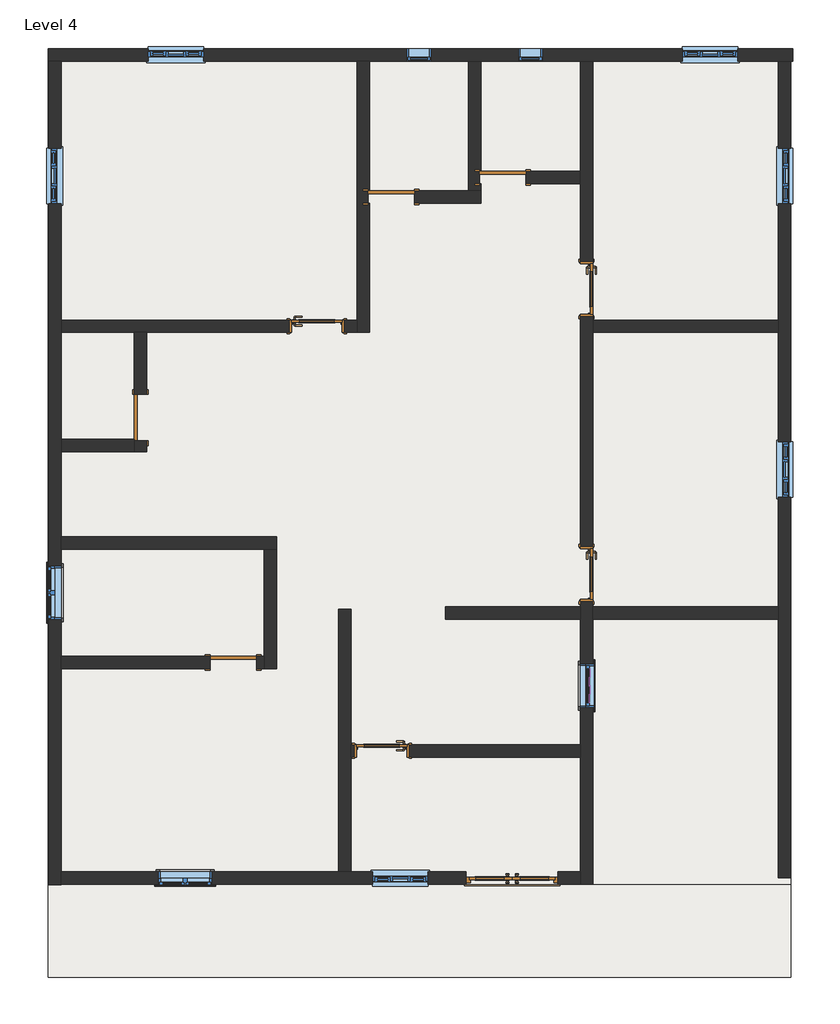
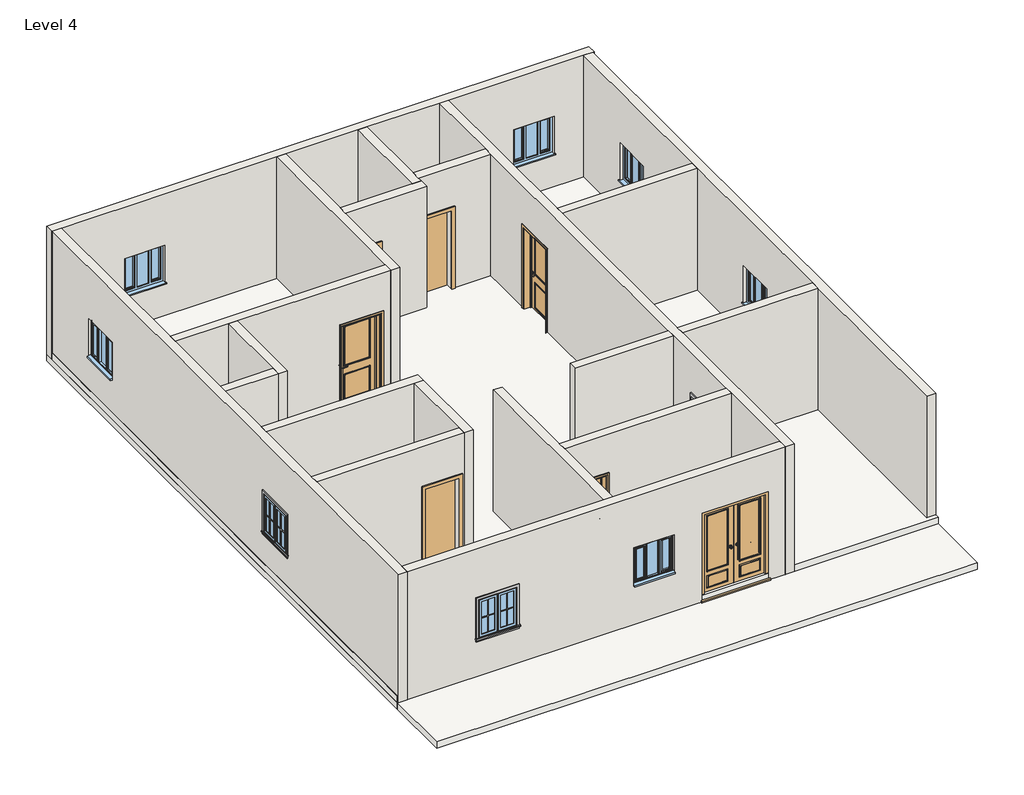
# One storey, incomplete: 19 walls, 12 proxies, 11 windows, 9 doors, 2 slabs, 1 roof.
"""IFC4 building model written with IfcOpenShell, lengths in millimetres."""

from ifc_helpers import new_model, si_unit, frame, origin, place, context, project, spatial, polyline, outline, extrude, faceted_brep, transform, mapped, element, save
from components import muntin_pattern_2x2_muntin_pattern_2x2_b3fe6957, muntin_pattern_2x2_muntin_pattern_2x2_3e0ecaf2, muntin_pattern_2x2_muntin_pattern_2x2_5f474966, trim_window_exterior_flat_with_sill_41619996, trim_window_exterior_flat_with_sill_68241f6a, trim_window_interior_flat_picture_frame_51c85655, trim_window_interior_flat_picture_frame_d3d93820, doors_extdbl_w_glazing_bars_2_1510x2110mm_e5cd3545, doors_extdbl_w_glazing_bars_2_1510x2110mm_b3535315, doors_intsgl_w_transome_910x2110mm_1071bad6, doors_intsgl_w_transome_910x2110mm_0d7ac49b, door_fadea3f2, door_53b1b562, window_085f26e1, window_c29befe5, window_4d695ea9, windows_tpl_plain_910x910mm_84e79c20

model = new_model("IFC4")

# Units and contexts
model_context = context("Model", 3, world=origin())
ifc_project = project(units=[si_unit("LENGTHUNIT", "METRE", prefix="MILLI")], contexts=[model_context])

# Site, building, storey
site = spatial("IfcSite", under=ifc_project)
building = spatial("IfcBuilding", under=site)
storey = spatial("IfcBuildingStorey", under=building, Name="Level 4", Elevation=9144.0)

# Proxies
placement = place(None, origin())
muntin_pattern_2x2_muntin_pattern_2x2_shape = muntin_pattern_2x2_muntin_pattern_2x2_b3fe6957(model_context)
element("IfcBuildingElementProxy", 1, Name="Muntin Pattern_2x2 : Muntin Pattern_2x2", ObjectType="Muntin Pattern_2x2 : Muntin Pattern_2x2", at=placement, inside=storey, context=model_context, shape_type="MappedRepresentation", body=[
    mapped(muntin_pattern_2x2_muntin_pattern_2x2_shape, transform((-4444.3565281, -6259.9254533, 10128.25), x_axis=(-1.0, 0.0, 0.0), y_axis=(0.0, -1.0, 0.0), z_axis=(0.0, 0.0, 1.0))),
])
element("IfcBuildingElementProxy", 2, Name="Muntin Pattern_2x2 : Muntin Pattern_2x2", ObjectType="Muntin Pattern_2x2 : Muntin Pattern_2x2", at=placement, inside=storey, context=model_context, shape_type="MappedRepresentation", body=[
    mapped(muntin_pattern_2x2_muntin_pattern_2x2_shape, transform((-6884.3440281, -1708.5629533, 10128.25), x_axis=(0.0, 1.0, 0.0), y_axis=(-1.0, 0.0, 0.0), z_axis=(0.0, 0.0, 1.0))),
])
muntin_pattern_2x2_muntin_pattern_2x2_2_shape = muntin_pattern_2x2_muntin_pattern_2x2_3e0ecaf2(model_context)
element("IfcBuildingElementProxy", 3, Name="Muntin Pattern_2x2 : Muntin Pattern_2x2", ObjectType="Muntin Pattern_2x2 : Muntin Pattern_2x2", at=placement, inside=storey, context=model_context, shape_type="MappedRepresentation", body=[
    mapped(muntin_pattern_2x2_muntin_pattern_2x2_2_shape, transform((-4872.9815281, -6259.9254533, 10128.25), x_axis=(1.0, 0.0, 0.0), y_axis=(0.0, 1.0, 0.0), z_axis=(0.0, 0.0, 1.0))),
])
element("IfcBuildingElementProxy", 4, Name="Muntin Pattern_2x2 : Muntin Pattern_2x2", ObjectType="Muntin Pattern_2x2 : Muntin Pattern_2x2", at=placement, inside=storey, context=model_context, shape_type="MappedRepresentation", body=[
    mapped(muntin_pattern_2x2_muntin_pattern_2x2_2_shape, transform((-6884.3440281, -1279.9379533, 10128.25), x_axis=(0.0, -1.0, 0.0), y_axis=(1.0, 0.0, 0.0), z_axis=(0.0, 0.0, 1.0))),
])
muntin_pattern_2x2_muntin_pattern_2x2_3_shape = muntin_pattern_2x2_muntin_pattern_2x2_5f474966(model_context)
element("IfcBuildingElementProxy", 5, Name="Muntin Pattern_2x2 : Muntin Pattern_2x2", ObjectType="Muntin Pattern_2x2 : Muntin Pattern_2x2", at=placement, inside=storey, context=model_context, shape_type="MappedRepresentation", body=[
    mapped(muntin_pattern_2x2_muntin_pattern_2x2_3_shape, transform((1989.809459, -3018.2504533, 10664.825), x_axis=(0.0, -1.0, 0.0), y_axis=(1.0, 0.0, 0.0), z_axis=(0.0, 0.0, 1.0))),
])
element("IfcBuildingElementProxy", 6, Name="Muntin Pattern_2x2 : Muntin Pattern_2x2", ObjectType="Muntin Pattern_2x2 : Muntin Pattern_2x2", at=placement, inside=storey, context=model_context, shape_type="MappedRepresentation", body=[
    mapped(muntin_pattern_2x2_muntin_pattern_2x2_3_shape, transform((1945.359459, -3018.2504533, 10134.6), x_axis=(0.0, -1.0, 0.0), y_axis=(1.0, 0.0, 0.0), z_axis=(0.0, 0.0, 1.0))),
])
trim_window_exterior_flat_with_sill_shape = trim_window_exterior_flat_with_sill_41619996(model_context)
element("IfcBuildingElementProxy", 7, Name="Trim-Window-Exterior-Flat : with Sill", ObjectType="Trim-Window-Exterior-Flat : with Sill", at=placement, inside=storey, context=model_context, shape_type="MappedRepresentation", body=[
    mapped(trim_window_exterior_flat_with_sill_shape, transform((-4658.6690281, -6269.4504533, 10972.8), x_axis=(1.0, 0.0, 0.0), y_axis=(0.0, 0.0, 1.0), z_axis=(0.0, -1.0, 0.0))),
])
element("IfcBuildingElementProxy", 8, Name="Trim-Window-Exterior-Flat : with Sill", ObjectType="Trim-Window-Exterior-Flat : with Sill", at=placement, inside=storey, context=model_context, shape_type="MappedRepresentation", body=[
    mapped(trim_window_exterior_flat_with_sill_shape, transform((-6893.8690281, -1494.2504533, 10972.8), x_axis=(0.0, -1.0, 0.0), y_axis=(0.0, 0.0, 1.0), z_axis=(-1.0, 0.0, 0.0))),
])
trim_window_exterior_flat_with_sill_2_shape = trim_window_exterior_flat_with_sill_68241f6a(model_context)
element("IfcBuildingElementProxy", 9, Name="Trim-Window-Exterior-Flat : with Sill", ObjectType="Trim-Window-Exterior-Flat : with Sill", at=placement, inside=storey, context=model_context, shape_type="MappedRepresentation", body=[
    mapped(trim_window_exterior_flat_with_sill_2_shape, transform((2024.734459, -3018.2504533, 11226.8), x_axis=(0.0, 1.0, 0.0), y_axis=(0.0, 0.0, 1.0), z_axis=(1.0, 0.0, 0.0))),
])
trim_window_interior_flat_picture_frame_shape = trim_window_interior_flat_picture_frame_51c85655(model_context)
element("IfcBuildingElementProxy", 10, Name="Trim-Window-Interior-Flat : Picture Frame", ObjectType="Trim-Window-Interior-Flat : Picture Frame", at=placement, inside=storey, context=model_context, shape_type="MappedRepresentation", body=[
    mapped(trim_window_interior_flat_picture_frame_shape, transform((-4658.6690281, -6066.2504533, 10972.8), x_axis=(-1.0, 0.0, 0.0), y_axis=(0.0, 0.0, 1.0), z_axis=(0.0, 1.0, 0.0))),
])
element("IfcBuildingElementProxy", 11, Name="Trim-Window-Interior-Flat : Picture Frame", ObjectType="Trim-Window-Interior-Flat : Picture Frame", at=placement, inside=storey, context=model_context, shape_type="MappedRepresentation", body=[
    mapped(trim_window_interior_flat_picture_frame_shape, transform((-6690.6690281, -1494.2504533, 10972.8), x_axis=(0.0, 1.0, 0.0), y_axis=(0.0, 0.0, 1.0), z_axis=(1.0, 0.0, 0.0))),
])
trim_window_interior_flat_picture_frame_2_shape = trim_window_interior_flat_picture_frame_d3d93820(model_context)
element("IfcBuildingElementProxy", 12, Name="Trim-Window-Interior-Flat : Picture Frame", ObjectType="Trim-Window-Interior-Flat : Picture Frame", at=placement, inside=storey, context=model_context, shape_type="MappedRepresentation", body=[
    mapped(trim_window_interior_flat_picture_frame_2_shape, transform((1821.534459, -3018.2504533, 11226.8), x_axis=(0.0, -1.0, 0.0), y_axis=(0.0, 0.0, 1.0), z_axis=(-1.0, 0.0, 0.0))),
])

# Doors
doors_extdbl_w_glazing_bars_2_1510x2110mm_shape = doors_extdbl_w_glazing_bars_2_1510x2110mm_e5cd3545(model_context)
doors_extdbl_w_glazing_bars_2_1510x2110mm_2_shape = doors_extdbl_w_glazing_bars_2_1510x2110mm_b3535315(model_context)
element("IfcDoor", 13, ObjectType="Doors_ExtDbl_w-Glazing_Bars_2 : 1510x2110mm", at=placement, inside=storey, context=model_context, shape_type="MappedRepresentation", body=[
    mapped(doors_extdbl_w_glazing_bars_2_1510x2110mm_shape, transform((703.934459, -6167.8504533, 9144.0), x_axis=(-1.0, 0.0, 0.0), y_axis=(0.0, -1.0, 0.0), z_axis=(0.0, 0.0, 1.0))),
    mapped(doors_extdbl_w_glazing_bars_2_1510x2110mm_2_shape, transform((703.934459, -6167.8504533, 9144.0), x_axis=(-1.0, 0.0, 0.0), y_axis=(0.0, -1.0, 0.0), z_axis=(0.0, 0.0, 1.0))),
])
doors_intsgl_w_transome_910x2110mm_shape = doors_intsgl_w_transome_910x2110mm_1071bad6(model_context)
element("IfcDoor", 14, ObjectType="Doors_IntSgl_w-Transome : 910x2110mm", at=placement, inside=storey, context=model_context, shape_type="MappedRepresentation", body=[
    mapped(doors_intsgl_w_transome_910x2110mm_shape, transform((-1432.8690281, -4085.0504533, 9144.0), x_axis=(-1.0, 0.0, 0.0), y_axis=(0.0, -1.0, 0.0), z_axis=(0.0, 0.0, 1.0))),
])
doors_intsgl_w_transome_910x2110mm_2_shape = doors_intsgl_w_transome_910x2110mm_0d7ac49b(model_context)
element("IfcDoor", 15, ObjectType="Doors_IntSgl_w-Transome : 910x2110mm", at=placement, inside=storey, context=model_context, shape_type="MappedRepresentation", body=[
    mapped(doors_intsgl_w_transome_910x2110mm_2_shape, transform((-2499.6690281, 2874.5495467, 9144.0), x_axis=(1.0, 0.0, 0.0), y_axis=(0.0, 1.0, 0.0), z_axis=(0.0, 0.0, 1.0))),
])
element("IfcDoor", 16, ObjectType="Doors_IntSgl_w-Transome : 910x2110mm", at=placement, inside=storey, context=model_context, shape_type="MappedRepresentation", body=[
    mapped(doors_intsgl_w_transome_910x2110mm_2_shape, transform((1923.134459, 3484.1495467, 9144.0), x_axis=(0.0, -1.0, 0.0), y_axis=(1.0, 0.0, 0.0), z_axis=(0.0, 0.0, 1.0))),
])
element("IfcDoor", 17, ObjectType="Doors_IntSgl_w-Transome : 910x2110mm", at=placement, inside=storey, context=model_context, shape_type="MappedRepresentation", body=[
    mapped(doors_intsgl_w_transome_910x2110mm_2_shape, transform((1923.134459, -1189.4504533, 9144.0), x_axis=(0.0, -1.0, 0.0), y_axis=(1.0, 0.0, 0.0), z_axis=(0.0, 0.0, 1.0))),
])
door_shape = door_fadea3f2(model_context)
element("IfcDoor", 18, ObjectType="Single-Flush : 30\" x 80\"", at=placement, inside=storey, context=model_context, shape_type="MappedRepresentation", body=[
    mapped(door_shape, transform((-3871.2690281, -2637.2504533, 9144.0), x_axis=(1.0, 0.0, 0.0), y_axis=(0.0, 1.0, 0.0), z_axis=(0.0, 0.0, 1.0))),
])
door_2_shape = door_53b1b562(model_context)
element("IfcDoor", 19, ObjectType="Single-Flush : 30\" x 80\"", at=placement, inside=storey, context=model_context, shape_type="MappedRepresentation", body=[
    mapped(door_2_shape, transform((-5395.2690281, 1375.9495467, 9144.0), x_axis=(0.0, -1.0, 0.0), y_axis=(1.0, 0.0, 0.0), z_axis=(0.0, 0.0, 1.0))),
])
element("IfcDoor", 20, ObjectType="Single-Flush : 30\" x 80\"", at=placement, inside=storey, context=model_context, shape_type="MappedRepresentation", body=[
    mapped(door_2_shape, transform((-1280.4690281, 4995.4495467, 9144.0), x_axis=(-1.0, 0.0, 0.0), y_axis=(0.0, -1.0, 0.0), z_axis=(0.0, 0.0, 1.0))),
])
element("IfcDoor", 21, ObjectType="Single-Flush : 30\" x 80\"", at=placement, inside=storey, context=model_context, shape_type="MappedRepresentation", body=[
    mapped(door_2_shape, transform((548.3309719, 5312.9495467, 9144.0), x_axis=(-1.0, 0.0, 0.0), y_axis=(0.0, -1.0, 0.0), z_axis=(0.0, 0.0, 1.0))),
])

# Roof
element("IfcRoof", 22, ObjectType="Generic - 12\"", at=placement, inside=storey, context=model_context, shape_type="SweptSolid", body=[
    extrude(outline(polyline([(-6906.5690281, 7421.1495467), (5272.7309719, 7421.1495467), (5272.7309719, -6269.4504533), (-6906.5690281, -6269.4504533), (-6906.5690281, 7421.1495467)])), frame((0.0, 0.0, 9144.0), z_axis=(0.0, 0.0, 1.0), x_axis=(1.0, 0.0, 0.0)), (0.0, 0.0, 1.0), 152.4),
])

# Slabs
element("IfcSlab", 23, ObjectType="Generic - 12\"", at=placement, inside=storey, context=model_context, shape_type="SweptSolid", body=[
    extrude(outline(polyline([(5272.7309719, 7421.1495467), (5272.7309719, -6269.4504533), (-6906.5690281, -6269.4504533), (-6906.5690281, 7421.1495467), (5272.7309719, 7421.1495467)])), frame((0.0, 0.0, 8991.6), z_axis=(0.0, 0.0, 1.0), x_axis=(1.0, 0.0, 0.0)), (0.0, 0.0, 1.0), 152.4),
])
element("IfcSlab", 24, ObjectType="Generic - 12\"", at=placement, inside=storey, context=model_context, shape_type="SweptSolid", body=[
    extrude(outline(polyline([(5272.7309719, -6269.4504533), (5272.7309719, -7799.0240652), (-6906.5690281, -7799.0240652), (-6906.5690281, -6269.4504533), (5272.7309719, -6269.4504533)])), frame((0.0, 0.0, 8991.6), z_axis=(0.0, 0.0, 1.0), x_axis=(1.0, 0.0, 0.0)), (0.0, 0.0, 1.0), 152.4),
])

# Walls
element("IfcWall", 25, ObjectType="4.5\" p", at=placement, inside=storey, context=model_context, shape_type="Brep", body=[
    faceted_brep([(-1839.2690281, 7217.9495467, 9144.0), (-1839.2690281, 2976.1495467, 9144.0), (-1839.2690281, 2772.9495467, 9144.0), (-1839.2690281, 2772.9495467, 12192.0), (-1839.2690281, 2976.1495467, 12192.0), (-1839.2690281, 7217.9495467, 12192.0), (-1636.0690281, 7217.9495467, 12192.0), (-1636.0690281, 5097.0495467, 12192.0), (-1636.0690281, 4893.8495467, 12192.0), (-1636.0690281, 2772.9495467, 12192.0), (-1636.0690281, 2772.9495467, 9144.0), (-1636.0690281, 4893.8495467, 9144.0), (-1636.0690281, 4893.8495467, 11176.0), (-1636.0690281, 5097.0495467, 11176.0), (-1636.0690281, 5097.0495467, 9144.0), (-1636.0690281, 7217.9495467, 9144.0), (-1661.4690281, 5097.0495467, 9144.0), (-1661.4690281, 4893.8495467, 9144.0), (-1661.4690281, 5097.0495467, 11176.0), (-1661.4690281, 4893.8495467, 11176.0)], [[[0, 1, 2, 3, 4, 5]], [[6, 7, 8, 9, 10, 11, 12, 13, 14, 15]], [[2, 1, 0, 15, 14, 16, 17, 11, 10]], [[5, 4, 3, 9, 8, 7, 6]], [[0, 5, 6, 15]], [[3, 2, 10, 9]], [[18, 16, 14, 13]], [[17, 19, 12, 11]], [[19, 18, 13, 12]], [[16, 18, 19, 17]]]),
])
element("IfcWall", 26, ObjectType="4.5\" p", at=placement, inside=storey, context=model_context, shape_type="Brep", body=[
    faceted_brep([(-1839.2690281, 2772.9495467, 12192.0), (-5293.6690281, 2772.9495467, 12192.0), (-5496.8690281, 2772.9495467, 12192.0), (-6690.6690281, 2772.9495467, 12192.0), (-6690.6690281, 2772.9495467, 9144.0), (-5496.8690281, 2772.9495467, 9144.0), (-5293.6690281, 2772.9495467, 9144.0), (-2954.6690281, 2772.9495467, 9144.0), (-2954.6690281, 2772.9495467, 11254.0), (-2044.6690281, 2772.9495467, 11254.0), (-2044.6690281, 2772.9495467, 9144.0), (-1839.2690281, 2772.9495467, 9144.0), (-6690.6690281, 2976.1495467, 12192.0), (-1839.2690281, 2976.1495467, 12192.0), (-1839.2690281, 2976.1495467, 9144.0), (-2044.6690281, 2976.1495467, 9144.0), (-2044.6690281, 2976.1495467, 11254.0), (-2954.6690281, 2976.1495467, 11254.0), (-2954.6690281, 2976.1495467, 9144.0), (-6690.6690281, 2976.1495467, 9144.0)], [[[0, 1, 2, 3, 4, 5, 6, 7, 8, 9, 10, 11]], [[12, 13, 14, 15, 16, 17, 18, 19]], [[4, 19, 18, 7, 6, 5]], [[14, 11, 10, 15]], [[3, 2, 1, 0, 13, 12]], [[0, 11, 14, 13]], [[4, 3, 12, 19]], [[9, 16, 15, 10]], [[16, 9, 8, 17]], [[17, 8, 7, 18]]]),
])
element("IfcWall", 27, ObjectType="4.5\" p", at=placement, inside=storey, context=model_context, shape_type="Brep", body=[
    faceted_brep([(-5496.8690281, 994.9495467, 11176.0), (-5496.8690281, 994.9495467, 9144.0), (-5496.8690281, 817.1495467, 9144.0), (-5496.8690281, 817.1495467, 12192.0), (-5496.8690281, 1020.3495467, 12192.0), (-5496.8690281, 2772.9495467, 12192.0), (-5496.8690281, 2772.9495467, 9144.0), (-5496.8690281, 1756.9495467, 9144.0), (-5496.8690281, 1756.9495467, 11176.0), (-5293.6690281, 817.1495467, 9144.0), (-5293.6690281, 994.9495467, 9144.0), (-5293.6690281, 994.9495467, 11176.0), (-5293.6690281, 1756.9495467, 11176.0), (-5293.6690281, 1756.9495467, 9144.0), (-5293.6690281, 2772.9495467, 9144.0), (-5293.6690281, 2772.9495467, 12192.0), (-5293.6690281, 817.1495467, 12192.0)], [[[0, 1, 2, 3, 4, 5, 6, 7, 8]], [[9, 10, 11, 12, 13, 14, 15, 16]], [[7, 6, 14, 13]], [[2, 1, 10, 9]], [[5, 4, 3, 16, 15]], [[6, 5, 15, 14]], [[3, 2, 9, 16]], [[11, 10, 1, 0]], [[12, 11, 0, 8]], [[13, 12, 8, 7]]]),
])
element("IfcWall", 28, ObjectType="4.5\" p", at=placement, inside=storey, context=model_context, shape_type="SweptSolid", body=[
    extrude(outline(polyline([(-5496.8690281, 817.1495467), (-6690.6690281, 817.1495467), (-6690.6690281, 1020.3495467), (-5496.8690281, 1020.3495467), (-5496.8690281, 817.1495467)])), frame((0.0, 0.0, 9144.0), z_axis=(0.0, 0.0, 1.0), x_axis=(1.0, 0.0, 0.0)), (0.0, 0.0, 1.0), 3048.0),
])
element("IfcWall", 29, ObjectType="4.5\" p", at=placement, inside=storey, context=model_context, shape_type="Brep", body=[
    faceted_brep([(-6690.6690281, -783.0504533, 9144.0), (-3363.2690281, -783.0504533, 9144.0), (-3160.0690281, -783.0504533, 9144.0), (-3160.0690281, -783.0504533, 12192.0), (-3363.2690281, -783.0504533, 12192.0), (-6690.6690281, -783.0504533, 12192.0), (-6690.6690281, -579.8504533, 9144.0), (-6690.6690281, -579.8504533, 12192.0), (-3160.0690281, -579.8504533, 12192.0), (-3160.0690281, -579.8504533, 9144.0)], [[[0, 1, 2, 3, 4, 5]], [[6, 7, 8, 9]], [[2, 1, 0, 6, 9]], [[5, 4, 3, 8, 7]], [[0, 5, 7, 6]], [[3, 2, 9, 8]]]),
])
element("IfcWall", 30, ObjectType="4.5\" p", at=placement, inside=storey, context=model_context, shape_type="Brep", body=[
    faceted_brep([(-3363.2690281, -783.0504533, 9144.0), (-3363.2690281, -2535.6504533, 9144.0), (-3363.2690281, -2738.8504533, 9144.0), (-3363.2690281, -2738.8504533, 12192.0), (-3363.2690281, -2535.6504533, 12192.0), (-3363.2690281, -783.0504533, 12192.0), (-3160.0690281, -783.0504533, 9144.0), (-3160.0690281, -783.0504533, 12192.0), (-3160.0690281, -2738.8504533, 12192.0), (-3160.0690281, -2738.8504533, 9144.0)], [[[0, 1, 2, 3, 4, 5]], [[6, 7, 8, 9]], [[2, 1, 0, 6, 9]], [[5, 4, 3, 8, 7]], [[0, 5, 7, 6]], [[3, 2, 9, 8]]]),
])
element("IfcWall", 31, ObjectType="4.5\" p", at=placement, inside=storey, context=model_context, shape_type="SweptSolid", body=[
    extrude(outline(polyline([(11176.0, -3490.2690281), (9144.0, -3490.2690281), (9144.0, -3363.2690281), (12192.0, -3363.2690281), (12192.0, -6690.6690281), (9144.0, -6690.6690281), (9144.0, -4252.2690281), (11176.0, -4252.2690281), (11176.0, -3490.2690281)])), frame((0.0, -2738.8504533, 0.0), z_axis=(0.0, 1.0, 0.0), x_axis=(0.0, 0.0, 1.0)), (0.0, 0.0, 1.0), 203.2),
])
element("IfcWall", 32, ObjectType="4.5\" p", at=placement, inside=storey, context=model_context, shape_type="Brep", body=[
    faceted_brep([(192.7309719, 4893.8495467, 12192.0), (-1636.0690281, 4893.8495467, 12192.0), (-1636.0690281, 4893.8495467, 11176.0), (-899.4690281, 4893.8495467, 11176.0), (-899.4690281, 4893.8495467, 9144.0), (192.7309719, 4893.8495467, 9144.0), (-1636.0690281, 5097.0495467, 12192.0), (-10.4690281, 5097.0495467, 12192.0), (192.7309719, 5097.0495467, 12192.0), (192.7309719, 5097.0495467, 9144.0), (-10.4690281, 5097.0495467, 9144.0), (-899.4690281, 5097.0495467, 9144.0), (-899.4690281, 5097.0495467, 11176.0), (-1636.0690281, 5097.0495467, 11176.0)], [[[0, 1, 2, 3, 4, 5]], [[6, 7, 8, 9, 10, 11, 12, 13]], [[9, 5, 4, 11, 10]], [[1, 0, 8, 7, 6]], [[1, 6, 13, 2]], [[0, 5, 9, 8]], [[12, 3, 2, 13]], [[3, 12, 11, 4]]]),
])
element("IfcWall", 33, ObjectType="4.5\" p", at=placement, inside=storey, context=model_context, shape_type="Brep", body=[
    faceted_brep([(-10.4690281, 7217.9495467, 9144.0), (-10.4690281, 5097.0495467, 9144.0), (-10.4690281, 5097.0495467, 12192.0), (-10.4690281, 7217.9495467, 12192.0), (192.7309719, 7217.9495467, 12192.0), (192.7309719, 5414.5495467, 12192.0), (192.7309719, 5211.3495467, 12192.0), (192.7309719, 5097.0495467, 12192.0), (192.7309719, 5097.0495467, 9144.0), (192.7309719, 5211.3495467, 9144.0), (192.7309719, 5211.3495467, 11176.0), (192.7309719, 5414.5495467, 11176.0), (192.7309719, 5414.5495467, 9144.0), (192.7309719, 7217.9495467, 9144.0), (167.3309719, 5414.5495467, 9144.0), (167.3309719, 5211.3495467, 9144.0), (167.3309719, 5414.5495467, 11176.0), (167.3309719, 5211.3495467, 11176.0)], [[[0, 1, 2, 3]], [[4, 5, 6, 7, 8, 9, 10, 11, 12, 13]], [[1, 0, 13, 12, 14, 15, 9, 8]], [[3, 2, 7, 6, 5, 4]], [[2, 1, 8, 7]], [[0, 3, 4, 13]], [[16, 14, 12, 11]], [[15, 17, 10, 9]], [[17, 16, 11, 10]], [[14, 16, 17, 15]]]),
])
element("IfcWall", 34, ObjectType="4.5\" p", at=placement, inside=storey, context=model_context, shape_type="Brep", body=[
    faceted_brep([(1821.534459, -6269.4504533, 12192.0), (1821.534459, -6066.2504533, 12192.0), (1821.534459, -4186.6504533, 12192.0), (1821.534459, -3983.4504533, 12192.0), (1821.534459, -1926.0504533, 12192.0), (1821.534459, -1722.8504533, 12192.0), (1821.534459, 5211.3495467, 12192.0), (1821.534459, 5414.5495467, 12192.0), (1821.534459, 7217.9495467, 12192.0), (1821.534459, 7217.9495467, 9144.0), (1821.534459, 5414.5495467, 9144.0), (1821.534459, 5211.3495467, 9144.0), (1821.534459, 3939.1495467, 9144.0), (1821.534459, 3939.1495467, 11254.0), (1821.534459, 3029.1495467, 11254.0), (1821.534459, 3029.1495467, 9144.0), (1821.534459, -734.4504533, 9144.0), (1821.534459, -734.4504533, 11254.0), (1821.534459, -1644.4504533, 11254.0), (1821.534459, -1644.4504533, 9144.0), (1821.534459, -1722.8504533, 9144.0), (1821.534459, -1926.0504533, 9144.0), (1821.534459, -3983.4504533, 9144.0), (1821.534459, -4186.6504533, 9144.0), (1821.534459, -6066.2504533, 9144.0), (1821.534459, -6269.4504533, 9144.0), (1821.534459, -2662.6504533, 11226.8), (1821.534459, -3373.8504533, 11226.8), (1821.534459, -3373.8504533, 10058.4), (1821.534459, -2662.6504533, 10058.4), (2024.734459, 7217.9495467, 12192.0), (2024.734459, 2976.1495467, 12192.0), (2024.734459, 2772.9495467, 12192.0), (2024.734459, -1722.8504533, 12192.0), (2024.734459, -1926.0504533, 12192.0), (2024.734459, -6269.4504533, 12192.0), (2024.734459, -6269.4504533, 9144.0), (2024.734459, -1926.0504533, 9144.0), (2024.734459, -1722.8504533, 9144.0), (2024.734459, -1644.4504533, 9144.0), (2024.734459, -1644.4504533, 11254.0), (2024.734459, -734.4504533, 11254.0), (2024.734459, -734.4504533, 9144.0), (2024.734459, 2772.9495467, 9144.0), (2024.734459, 2976.1495467, 9144.0), (2024.734459, 3029.1495467, 9144.0), (2024.734459, 3029.1495467, 11254.0), (2024.734459, 3939.1495467, 11254.0), (2024.734459, 3939.1495467, 9144.0), (2024.734459, 7217.9495467, 9144.0), (2024.734459, -2662.6504533, 11226.8), (2024.734459, -2662.6504533, 10058.4), (2024.734459, -3373.8504533, 10058.4), (2024.734459, -3373.8504533, 11226.8)], [[[0, 1, 2, 3, 4, 5, 6, 7, 8, 9, 10, 11, 12, 13, 14, 15, 16, 17, 18, 19, 20, 21, 22, 23, 24, 25], [26, 27, 28, 29]], [[30, 31, 32, 33, 34, 35, 36, 37, 38, 39, 40, 41, 42, 43, 44, 45, 46, 47, 48, 49], [50, 51, 52, 53]], [[9, 49, 48, 12, 11, 10]], [[15, 45, 44, 43, 42, 16]], [[36, 25, 24, 23, 22, 21, 20, 19, 39, 38, 37]], [[8, 7, 6, 5, 4, 3, 2, 1, 0, 35, 34, 33, 32, 31, 30]], [[9, 8, 30, 49]], [[14, 46, 45, 15]], [[46, 14, 13, 47]], [[47, 13, 12, 48]], [[18, 40, 39, 19]], [[40, 18, 17, 41]], [[41, 17, 16, 42]], [[0, 25, 36, 35]], [[51, 50, 26, 29]], [[52, 51, 29, 28]], [[53, 52, 28, 27]], [[50, 53, 27, 26]]]),
])
element("IfcWall", 35, ObjectType="4.5\" p", at=placement, inside=storey, context=model_context, shape_type="SweptSolid", body=[
    extrude(outline(polyline([(-391.4690281, -1926.0504533), (-391.4690281, -1722.8504533), (1821.534459, -1722.8504533), (1821.534459, -1926.0504533), (-391.4690281, -1926.0504533)])), frame((0.0, 0.0, 9144.0), z_axis=(0.0, 0.0, 1.0), x_axis=(1.0, 0.0, 0.0)), (0.0, 0.0, 1.0), 3048.0),
    extrude(outline(polyline([(5069.5309719, -1722.8504533), (5069.5309719, -1926.0504533), (2024.734459, -1926.0504533), (2024.734459, -1722.8504533), (5069.5309719, -1722.8504533)])), frame((0.0, 0.0, 9144.0), z_axis=(0.0, 0.0, 1.0), x_axis=(1.0, 0.0, 0.0)), (0.0, 0.0, 1.0), 3048.0),
])
element("IfcWall", 36, ObjectType="4.5\" p", at=placement, inside=storey, context=model_context, shape_type="SweptSolid", body=[
    extrude(outline(polyline([(5069.5309719, 2772.9495467), (2024.734459, 2772.9495467), (2024.734459, 2976.1495467), (5069.5309719, 2976.1495467), (5069.5309719, 2772.9495467)])), frame((0.0, 0.0, 9144.0), z_axis=(0.0, 0.0, 1.0), x_axis=(1.0, 0.0, 0.0)), (0.0, 0.0, 1.0), 3048.0),
])
element("IfcWall", 37, ObjectType="4.5\" p", at=placement, inside=storey, context=model_context, shape_type="SweptSolid", body=[
    extrude(outline(polyline([(12192.0, 1821.534459), (12192.0, 192.7309719), (11176.0, 192.7309719), (11176.0, 929.3309719), (9144.0, 929.3309719), (9144.0, 1821.534459), (12192.0, 1821.534459)])), frame((0.0, 5211.3495467, 0.0), z_axis=(0.0, 1.0, 0.0), x_axis=(0.0, 0.0, 1.0)), (0.0, 0.0, 1.0), 203.2),
])
element("IfcWall", 38, ObjectType="4.5\" p", at=placement, inside=storey, context=model_context, shape_type="Brep", body=[
    faceted_brep([(-1940.8690281, -6066.2504533, 9144.0), (-1940.8690281, -4186.6504533, 9144.0), (-1940.8690281, -3983.4504533, 9144.0), (-1940.8690281, -1760.9504533, 9144.0), (-1940.8690281, -1760.9504533, 12192.0), (-1940.8690281, -3983.4504533, 12192.0), (-1940.8690281, -4186.6504533, 12192.0), (-1940.8690281, -6066.2504533, 12192.0), (-2144.0690281, -6066.2504533, 9144.0), (-2144.0690281, -6066.2504533, 12192.0), (-2144.0690281, -1760.9504533, 12192.0), (-2144.0690281, -1760.9504533, 9144.0)], [[[0, 1, 2, 3, 4, 5, 6, 7]], [[8, 9, 10, 11]], [[3, 2, 1, 0, 8, 11]], [[4, 3, 11, 10]], [[7, 6, 5, 4, 10, 9]], [[0, 7, 9, 8]]]),
])
element("IfcWall", 39, ObjectType="4.5\" p", at=placement, inside=storey, context=model_context, shape_type="SweptSolid", body=[
    extrude(outline(polyline([(12192.0, 1821.534459), (12192.0, -1940.8690281), (9144.0, -1940.8690281), (9144.0, -1887.8690281), (11254.0, -1887.8690281), (11254.0, -977.8690281), (9144.0, -977.8690281), (9144.0, 1821.534459), (12192.0, 1821.534459)])), frame((0.0, -4186.6504533, 0.0), z_axis=(0.0, 1.0, 0.0), x_axis=(0.0, 0.0, 1.0)), (0.0, 0.0, 1.0), 203.2),
])
element("IfcWall", 40, ObjectType="9\"", at=placement, inside=storey, context=model_context, shape_type="Brep", body=[
    faceted_brep([(5069.5309719, 7217.9495467, 9144.0), (5069.5309719, 2976.1495467, 9144.0), (5069.5309719, 2772.9495467, 9144.0), (5069.5309719, -1722.8504533, 9144.0), (5069.5309719, -1926.0504533, 9144.0), (5069.5309719, -6167.8504533, 9144.0), (5069.5309719, -6167.8504533, 12192.0), (5069.5309719, -1926.0504533, 12192.0), (5069.5309719, -1722.8504533, 12192.0), (5069.5309719, 2772.9495467, 12192.0), (5069.5309719, 2976.1495467, 12192.0), (5069.5309719, 7217.9495467, 12192.0), (5069.5309719, 980.0495467, 10968.4), (5069.5309719, 70.0495467, 10968.4), (5069.5309719, 70.0495467, 10058.4), (5069.5309719, 980.0495467, 10058.4), (5069.5309719, 5793.3495467, 10968.4), (5069.5309719, 4883.3495467, 10968.4), (5069.5309719, 4883.3495467, 10058.4), (5069.5309719, 5793.3495467, 10058.4), (5272.7309719, 7217.9495467, 9144.0), (5272.7309719, 7217.9495467, 12192.0), (5272.7309719, -6167.8504533, 12192.0), (5272.7309719, -6167.8504533, 9144.0), (5272.7309719, 980.0495467, 10968.4), (5272.7309719, 980.0495467, 10058.4), (5272.7309719, 70.0495467, 10058.4), (5272.7309719, 70.0495467, 10968.4), (5272.7309719, 5793.3495467, 10968.4), (5272.7309719, 5793.3495467, 10058.4), (5272.7309719, 4883.3495467, 10058.4), (5272.7309719, 4883.3495467, 10968.4)], [[[0, 1, 2, 3, 4, 5, 6, 7, 8, 9, 10, 11], [12, 13, 14, 15], [16, 17, 18, 19]], [[20, 21, 22, 23], [24, 25, 26, 27], [28, 29, 30, 31]], [[5, 4, 3, 2, 1, 0, 20, 23]], [[6, 5, 23, 22]], [[11, 10, 9, 8, 7, 6, 22, 21]], [[0, 11, 21, 20]], [[25, 24, 12, 15]], [[26, 25, 15, 14]], [[27, 26, 14, 13]], [[24, 27, 13, 12]], [[29, 28, 16, 19]], [[30, 29, 19, 18]], [[31, 30, 18, 17]], [[28, 31, 17, 16]]]),
])
element("IfcWall", 41, ObjectType="9\" wall", at=placement, inside=storey, context=model_context, shape_type="Brep", body=[
    faceted_brep([(-6906.5690281, 7217.9495467, 9144.0), (-6893.8690281, 7217.9495467, 9144.0), (-6690.6690281, 7217.9495467, 9144.0), (-1839.2690281, 7217.9495467, 9144.0), (-1636.0690281, 7217.9495467, 9144.0), (-10.4690281, 7217.9495467, 9144.0), (192.7309719, 7217.9495467, 9144.0), (1821.534459, 7217.9495467, 9144.0), (2024.734459, 7217.9495467, 9144.0), (5069.5309719, 7217.9495467, 9144.0), (5272.7309719, 7217.9495467, 9144.0), (5310.8309719, 7217.9495467, 9144.0), (5310.8309719, 7217.9495467, 12192.0), (5272.7309719, 7217.9495467, 12192.0), (5069.5309719, 7217.9495467, 12192.0), (2024.734459, 7217.9495467, 12192.0), (1821.534459, 7217.9495467, 12192.0), (192.7309719, 7217.9495467, 12192.0), (-10.4690281, 7217.9495467, 12192.0), (-1636.0690281, 7217.9495467, 12192.0), (-1839.2690281, 7217.9495467, 12192.0), (-6690.6690281, 7217.9495467, 12192.0), (-6893.8690281, 7217.9495467, 12192.0), (-6906.5690281, 7217.9495467, 12192.0), (-5266.0690281, 7217.9495467, 10968.4), (-4356.0690281, 7217.9495467, 10968.4), (-4356.0690281, 7217.9495467, 10058.4), (-5266.0690281, 7217.9495467, 10058.4), (3496.9309719, 7217.9495467, 10968.4), (4406.9309719, 7217.9495467, 10968.4), (4406.9309719, 7217.9495467, 10058.4), (3496.9309719, 7217.9495467, 10058.4), (-1026.4690281, 7217.9495467, 10668.0), (-620.0690281, 7217.9495467, 10668.0), (-620.0690281, 7217.9495467, 10058.4), (-1026.4690281, 7217.9495467, 10058.4), (803.9327155, 7217.9495467, 10668.0), (1210.3327155, 7217.9495467, 10668.0), (1210.3327155, 7217.9495467, 10058.4), (803.9327155, 7217.9495467, 10058.4), (-6906.5690281, 7421.1495467, 9144.0), (-6906.5690281, 7421.1495467, 12192.0), (5310.8309719, 7421.1495467, 12192.0), (5310.8309719, 7421.1495467, 9144.0), (-5266.0690281, 7421.1495467, 10968.4), (-5266.0690281, 7421.1495467, 10058.4), (-4356.0690281, 7421.1495467, 10058.4), (-4356.0690281, 7421.1495467, 10968.4), (3496.9309719, 7421.1495467, 10968.4), (3496.9309719, 7421.1495467, 10058.4), (4406.9309719, 7421.1495467, 10058.4), (4406.9309719, 7421.1495467, 10968.4), (-1026.4690281, 7421.1495467, 10668.0), (-1026.4690281, 7421.1495467, 10058.4), (-620.0690281, 7421.1495467, 10058.4), (-620.0690281, 7421.1495467, 10668.0), (803.9327155, 7421.1495467, 10668.0), (803.9327155, 7421.1495467, 10058.4), (1210.3327155, 7421.1495467, 10058.4), (1210.3327155, 7421.1495467, 10668.0)], [[[0, 1, 2, 3, 4, 5, 6, 7, 8, 9, 10, 11, 12, 13, 14, 15, 16, 17, 18, 19, 20, 21, 22, 23], [24, 25, 26, 27], [28, 29, 30, 31], [32, 33, 34, 35], [36, 37, 38, 39]], [[40, 41, 42, 43], [44, 45, 46, 47], [48, 49, 50, 51], [52, 53, 54, 55], [56, 57, 58, 59]], [[11, 10, 9, 8, 7, 6, 5, 4, 3, 2, 1, 0, 40, 43]], [[12, 11, 43, 42]], [[23, 22, 21, 20, 19, 18, 17, 16, 15, 14, 13, 12, 42, 41]], [[0, 23, 41, 40]], [[45, 44, 24, 27]], [[46, 45, 27, 26]], [[47, 46, 26, 25]], [[44, 47, 25, 24]], [[49, 48, 28, 31]], [[50, 49, 31, 30]], [[51, 50, 30, 29]], [[48, 51, 29, 28]], [[53, 52, 32, 35]], [[54, 53, 35, 34]], [[55, 54, 34, 33]], [[52, 55, 33, 32]], [[57, 56, 36, 39]], [[58, 57, 39, 38]], [[59, 58, 38, 37]], [[56, 59, 37, 36]]]),
])
element("IfcWall", 42, ObjectType="9\" wall", at=placement, inside=storey, context=model_context, shape_type="Brep", body=[
    faceted_brep([(-6893.8690281, 7217.9495467, 9144.0), (-6893.8690281, -6282.1504533, 9144.0), (-6893.8690281, -6282.1504533, 12192.0), (-6893.8690281, 7217.9495467, 12192.0), (-6893.8690281, -1062.4504533, 10972.8), (-6893.8690281, -1926.0504533, 10972.8), (-6893.8690281, -1926.0504533, 10058.4), (-6893.8690281, -1062.4504533, 10058.4), (-6893.8690281, 4883.3495467, 10968.4), (-6893.8690281, 4883.3495467, 10058.4), (-6893.8690281, 5793.3495467, 10058.4), (-6893.8690281, 5793.3495467, 10968.4), (-6690.6690281, 7217.9495467, 9144.0), (-6690.6690281, 7217.9495467, 12192.0), (-6690.6690281, 2976.1495467, 12192.0), (-6690.6690281, 2772.9495467, 12192.0), (-6690.6690281, 1020.3495467, 12192.0), (-6690.6690281, 817.1495467, 12192.0), (-6690.6690281, -579.8504533, 12192.0), (-6690.6690281, -783.0504533, 12192.0), (-6690.6690281, -2535.6504533, 12192.0), (-6690.6690281, -2738.8504533, 12192.0), (-6690.6690281, -6066.2504533, 12192.0), (-6690.6690281, -6269.4504533, 12192.0), (-6690.6690281, -6282.1504533, 12192.0), (-6690.6690281, -6282.1504533, 9144.0), (-6690.6690281, -6269.4504533, 9144.0), (-6690.6690281, -6066.2504533, 9144.0), (-6690.6690281, -2738.8504533, 9144.0), (-6690.6690281, -2535.6504533, 9144.0), (-6690.6690281, -783.0504533, 9144.0), (-6690.6690281, -579.8504533, 9144.0), (-6690.6690281, 817.1495467, 9144.0), (-6690.6690281, 1020.3495467, 9144.0), (-6690.6690281, 2772.9495467, 9144.0), (-6690.6690281, 2976.1495467, 9144.0), (-6690.6690281, -1062.4504533, 10972.8), (-6690.6690281, -1062.4504533, 10058.4), (-6690.6690281, -1926.0504533, 10058.4), (-6690.6690281, -1926.0504533, 10972.8), (-6690.6690281, 4883.3495467, 10968.4), (-6690.6690281, 5793.3495467, 10968.4), (-6690.6690281, 5793.3495467, 10058.4), (-6690.6690281, 4883.3495467, 10058.4)], [[[0, 1, 2, 3], [4, 5, 6, 7], [8, 9, 10, 11]], [[12, 13, 14, 15, 16, 17, 18, 19, 20, 21, 22, 23, 24, 25, 26, 27, 28, 29, 30, 31, 32, 33, 34, 35], [36, 37, 38, 39], [40, 41, 42, 43]], [[1, 0, 12, 35, 34, 33, 32, 31, 30, 29, 28, 27, 26, 25]], [[2, 1, 25, 24]], [[3, 2, 24, 23, 22, 21, 20, 19, 18, 17, 16, 15, 14, 13]], [[0, 3, 13, 12]], [[37, 36, 4, 7]], [[38, 37, 7, 6]], [[39, 38, 6, 5]], [[36, 39, 5, 4]], [[9, 8, 40, 43]], [[10, 9, 43, 42]], [[11, 10, 42, 41]], [[8, 11, 41, 40]]]),
])
element("IfcWall", 43, ObjectType="9\" wall", at=placement, inside=storey, context=model_context, shape_type="Brep", body=[
    faceted_brep([(1821.534459, -6269.4504533, 12192.0), (-6690.6690281, -6269.4504533, 12192.0), (-6690.6690281, -6269.4504533, 9144.0), (-51.065541, -6269.4504533, 9144.0), (-51.065541, -6269.4504533, 11254.0), (1458.934459, -6269.4504533, 11254.0), (1458.934459, -6269.4504533, 9144.0), (1821.534459, -6269.4504533, 9144.0), (-5090.4690281, -6269.4504533, 10972.8), (-4226.8690281, -6269.4504533, 10972.8), (-4226.8690281, -6269.4504533, 10058.4), (-5090.4690281, -6269.4504533, 10058.4), (-673.0690281, -6269.4504533, 10968.4), (-673.0690281, -6269.4504533, 10058.4), (-1583.0690281, -6269.4504533, 10058.4), (-1583.0690281, -6269.4504533, 10968.4), (-6690.6690281, -6066.2504533, 12192.0), (-2144.0690281, -6066.2504533, 12192.0), (-1940.8690281, -6066.2504533, 12192.0), (1821.534459, -6066.2504533, 12192.0), (1821.534459, -6066.2504533, 9144.0), (1458.934459, -6066.2504533, 9144.0), (1458.934459, -6066.2504533, 11254.0), (-51.065541, -6066.2504533, 11254.0), (-51.065541, -6066.2504533, 9144.0), (-1940.8690281, -6066.2504533, 9144.0), (-2144.0690281, -6066.2504533, 9144.0), (-6690.6690281, -6066.2504533, 9144.0), (-5090.4690281, -6066.2504533, 10972.8), (-5090.4690281, -6066.2504533, 10058.4), (-4226.8690281, -6066.2504533, 10058.4), (-4226.8690281, -6066.2504533, 10972.8), (-673.0690281, -6066.2504533, 10968.4), (-1583.0690281, -6066.2504533, 10968.4), (-1583.0690281, -6066.2504533, 10058.4), (-673.0690281, -6066.2504533, 10058.4)], [[[0, 1, 2, 3, 4, 5, 6, 7], [8, 9, 10, 11], [12, 13, 14, 15]], [[16, 17, 18, 19, 20, 21, 22, 23, 24, 25, 26, 27], [28, 29, 30, 31], [32, 33, 34, 35]], [[20, 7, 6, 21]], [[2, 27, 26, 25, 24, 3]], [[1, 0, 19, 18, 17, 16]], [[0, 7, 20, 19]], [[2, 1, 16, 27]], [[29, 28, 8, 11]], [[30, 29, 11, 10]], [[31, 30, 10, 9]], [[28, 31, 9, 8]], [[5, 22, 21, 6]], [[22, 5, 4, 23]], [[23, 4, 3, 24]], [[13, 12, 32, 35]], [[14, 13, 35, 34]], [[15, 14, 34, 33]], [[12, 15, 33, 32]]]),
])

# Windows
window_shape = window_085f26e1(model_context)
element("IfcWindow", 44, ObjectType="Fixed : 16\" x 24\"", at=placement, inside=storey, context=model_context, shape_type="MappedRepresentation", body=[
    mapped(window_shape, transform((-861.3690281, 7319.5495467, 9144.0), x_axis=(-1.0, 0.0, 0.0), y_axis=(0.0, -1.0, 0.0), z_axis=(0.0, 0.0, 1.0))),
])
element("IfcWindow", 45, ObjectType="Fixed : 16\" x 24\"", at=placement, inside=storey, context=model_context, shape_type="MappedRepresentation", body=[
    mapped(window_shape, transform((969.0327155, 7319.5495467, 9144.0), x_axis=(-1.0, 0.0, 0.0), y_axis=(0.0, -1.0, 0.0), z_axis=(0.0, 0.0, 1.0))),
])
window_2_shape = window_c29befe5(model_context)
element("IfcWindow", 46, ObjectType="Window-Casement-Double : 34\" x 36\"", at=placement, inside=storey, context=model_context, shape_type="MappedRepresentation", body=[
    mapped(window_2_shape, transform((-4658.6690281, -6167.8504533, 9144.0), x_axis=(-1.0, 0.0, 0.0), y_axis=(0.0, -1.0, 0.0), z_axis=(0.0, 0.0, 1.0))),
])
element("IfcWindow", 47, ObjectType="Window-Casement-Double : 34\" x 36\"", at=placement, inside=storey, context=model_context, shape_type="MappedRepresentation", body=[
    mapped(window_2_shape, transform((-6792.2690281, -1494.2504533, 9144.0), x_axis=(0.0, 1.0, 0.0), y_axis=(-1.0, 0.0, 0.0), z_axis=(0.0, 0.0, 1.0))),
])
window_3_shape = window_4d695ea9(model_context)
element("IfcWindow", 48, ObjectType="Window-Double-Hung : 28\" x 46\"", at=placement, inside=storey, context=model_context, shape_type="MappedRepresentation", body=[
    mapped(window_3_shape, transform((1923.134459, -3018.2504533, 9144.0), x_axis=(0.0, -1.0, 0.0), y_axis=(1.0, 0.0, 0.0), z_axis=(0.0, 0.0, 1.0))),
])
windows_tpl_plain_910x910mm_shape = windows_tpl_plain_910x910mm_84e79c20(model_context)
element("IfcWindow", 49, ObjectType="Windows_Tpl_Plain : 910x910mm", at=placement, inside=storey, context=model_context, shape_type="MappedRepresentation", body=[
    mapped(windows_tpl_plain_910x910mm_shape, transform((-1554.7356948, -6159.3938855, 8858.4), x_axis=(-1.0, 0.0, 0.0), y_axis=(0.0, -1.0, 0.0), z_axis=(0.0, 0.0, 1.0))),
])
element("IfcWindow", 50, ObjectType="Windows_Tpl_Plain : 910x910mm", at=placement, inside=storey, context=model_context, shape_type="MappedRepresentation", body=[
    mapped(windows_tpl_plain_910x910mm_shape, transform((-6783.8124603, 5765.0162133, 8858.4), x_axis=(0.0, 1.0, 0.0), y_axis=(-1.0, 0.0, 0.0), z_axis=(0.0, 0.0, 1.0))),
])
element("IfcWindow", 51, ObjectType="Windows_Tpl_Plain : 910x910mm", at=placement, inside=storey, context=model_context, shape_type="MappedRepresentation", body=[
    mapped(windows_tpl_plain_910x910mm_shape, transform((-4384.4023614, 7311.0929788, 8858.4), x_axis=(1.0, 0.0, 0.0), y_axis=(0.0, 1.0, 0.0), z_axis=(0.0, 0.0, 1.0))),
])
element("IfcWindow", 52, ObjectType="Windows_Tpl_Plain : 910x910mm", at=placement, inside=storey, context=model_context, shape_type="MappedRepresentation", body=[
    mapped(windows_tpl_plain_910x910mm_shape, transform((4378.5976386, 7311.0929788, 8858.4), x_axis=(1.0, 0.0, 0.0), y_axis=(0.0, 1.0, 0.0), z_axis=(0.0, 0.0, 1.0))),
])
element("IfcWindow", 53, ObjectType="Windows_Tpl_Plain : 910x910mm", at=placement, inside=storey, context=model_context, shape_type="MappedRepresentation", body=[
    mapped(windows_tpl_plain_910x910mm_shape, transform((5162.6744041, 98.38288, 8858.4), x_axis=(0.0, -1.0, 0.0), y_axis=(1.0, 0.0, 0.0), z_axis=(0.0, 0.0, 1.0))),
])
element("IfcWindow", 54, ObjectType="Windows_Tpl_Plain : 910x910mm", at=placement, inside=storey, context=model_context, shape_type="MappedRepresentation", body=[
    mapped(windows_tpl_plain_910x910mm_shape, transform((5162.6744041, 4911.68288, 8858.4), x_axis=(0.0, -1.0, 0.0), y_axis=(1.0, 0.0, 0.0), z_axis=(0.0, 0.0, 1.0))),
])

save(model, "model.ifc")

# Revit data of these elements
# Type "Muntin Pattern_2x2 : Muntin Pattern_2x2"
#   Width [instance default] = 4' - 0"
#   Thickness = 0' - 0 1/2"
#   Height [instance default] = 4' - 0"
#   Distance = 0' - 0 3/4"
#   Interior Material [instance default] = none
#   Exterior Material [instance default] = none
#   Default Elevation = 0
# Type "Trim-Window-Exterior-Flat : with Sill"
#   Trim Width = 0' - 2 1/4"
#   Trim Thickness_Picture Frame = 0' - 1 1/4"
#   Trim Thickness_with Sill = 0' - 0 3/4"
#   Sill Thickness = 0' - 1 1/4"
#   Opening Width [instance default] = 2' - 0"
#   Opening Height [instance default] = 3' - 0"
#   Default Elevation = 4' - 0"
#   Sill = yes
#   Picture Frame = no
#   Trim Material [instance default] = none
# Type "Trim-Window-Interior-Flat : Picture Frame"
#   Trim Thickness_Picture Frame = 0' - 1 1/4"
#   Trim Width = 0' - 2 1/4"
#   Trim Thickness_with Sill = 0' - 0 3/4"
#   Sill Thickness = 0' - 1 1/4"
#   Opening Width [instance default] = 2' - 0"
#   Opening Height [instance default] = 3' - 0"
#   Default Elevation = 4' - 0"
#   Sill = no
#   Picture Frame = yes
#   Trim Material [instance default] = none
# Type "Doors_ExtDbl_w-Glazing_Bars_2 : 1510x2110mm"
#   Type Mark = "15"
#   Type Comments = "External Double"
#   Operation = "DoubleDoorSingleSwing"
#   Construction Type Id = "GSP4R"
#   Keynote = "L20"
#   Analytic Construction = "1/8 in Pilkington single glazing"
#   Wrap Layers (Int) from Ext = 0' - 6.98819"
#   Wrap Layers (Ext) from Ext = 0' - 4.03543"
#   Visual Light Transmittance = 0.9
#   Top of Intermediate Rail = 1' - 10.6378"
#   Thickness = 0' - 1.73228"
#   Stile Shutting = 0' - 4.92126"
#   Stile - Top Rail = 0' - 3.93701"
#   Stile - Lock Rail = 0' - 3.93701"
#   Stile - Hanging = 0' - 3.93701"
#   Stile - Bottom Rail = 0' - 6.88976"
#   Solar Heat Gain Coefficient = 0.78
#   Rough Width = 4' - 11.44882"
#   Rough Height = 6' - 11.07087"
#   O/A Frame Width = 0' - 2.51969"
#   Heat Transfer Coefficient (U) = 0.6496 BTU/(h·ft²·°F)
#   Handle Z Distance = 3' - 5.33858"
#   Glazing Thickness = 0' - 0.94488"
#   Glazing Bar Thickness = 0' - 0.7874"
#   FrameWidth = 0' - 1.65354"
#   FrameOffset - External = 0' - 0.98425"
#   FrameDepth = 0' - 3.50394"
#   Door Panel Width = 2' - 3.6378"
#   Door Panel Thickness = 0' - 1.73228"
#   Door Panel Height = 6' - 6.74016"
#   Cill Thickness = 0' - 2.14567"
#   Cill Projection = 0' - 1.1811"
#   Handle X Distance = 0' - 2.95276"
#   Height = 6' - 11.07087"
#   Structural Tolerance = 0' - 0.25591"
#   Tolerance = 0' - 0.11811"
#   Undercut = 0' - 0.15748"
#   Width = 4' - 11.44882"
#   Cill Extension = 0' - 0.98425"
#   Cavity Closer Width = 0' - 1.9685"
#   Cavity Closer Offset from Ext = 0' - 4.03543"
#   Cavity Closer Depth = 0' - 3.34646"
#   Vis - Ironmongery = yes
#   Vis - Glazing Bars = yes
#   Vis - Cavity Closers = yes
#   Define Thermal Properties by = 1
#   Function = 1
#   Material Glazing Bars = Door - Panel
#   Material Glass = Door - Glazing
#   Material Door = Door - Panel
#   Material Frame = Door - Frame/Mullion
#   Material Ironmongery = Door - Handle
#   Wall Closure = (empty or 0)
#   Assembly Code = ""
# Type "Doors_IntSgl_w-Transome : 910x2110mm"
#   Type Mark = "11"
#   Type Comments = "Internal Single"
#   Construction Type Id = "SGL"
#   Manufacturer = "Revit"
#   Keynote = "L20"
#   Description = "Internal Single Door"
#   Analytic Construction = "Large single-glazed windows"
#   Visual Light Transmittance = 0.9
#   UnderCut = 0' - 0.31496"
#   Top of Lock Rail = 3' - 3.37008"
#   Tolerance = 0' - 0.07874"
#   Thickness = 0' - 1.49606"
#   Structural Tolerance = 0' - 0.31496"
#   StopDepth = 0' - 1.25984"
#   Stop Thickness = 0' - 0.74803"
#   Stile Top Rail = 0' - 4.92126"
#   Stile Shutting = 0' - 4.92126"
#   Stile Lock Rail = 0' - 7.87402"
#   Stile Hanging = 0' - 4.92126"
#   Stile Bottom Rail = 0' - 7.87402"
#   Solar Heat Gain Coefficient = 0.86
#   Rough Width = 2' - 11.82677"
#   Rough Height = 6' - 11.07087"
#   Height to Top Lock Rail = 3' - 3.37008"
#   Heat Transfer Coefficient (U) = 0.979472 BTU/(h·ft²·°F)
#   Handle Z Distance = 3' - 3.37008"
#   Handle X Distance = 0' - 1.9685"
#   Frame Thickness = 0' - 1.25984"
#   Door Panel Width = 2' - 8.51969"
#   Door Panel Thickness = 0' - 1.49606"
#   Door Panel Offset = 0' - 0"
#   Height = 6' - 11.07087"
#   Width = 2' - 11.82677"
#   Door Panel Height = 6' - 9.10236"
#   Architrave Setback = 0' - 0.19685"
#   Vis - Ironmongery = yes
#   Define Thermal Properties by = 1
#   Material Ironmongery = Door - Handle
#   Material Glass = Door - Glazing
#   Material Frame = Door - Frame/Mullion
#   Material Door = Door - Panel
#   Material Beading = Door - Panel
#   Material Architrave = Door - Architrave
#   Function = (empty or 0)
#   Wall Closure = (empty or 0)
# Type "Single-Flush : 30\" x 80\""
#   Type Mark = "5"
#   Construction Type Id = "MDOOR"
#   Assembly Code = "C1020"
#   Analytic Construction = "Metal"
#   Thickness = 0' - 2"
#   Heat Transfer Coefficient (U) = 0.651978 BTU/(h·ft²·°F)
#   Height = 6' - 8"
#   Trim Projection Ext = 0' - 1"
#   Trim Projection Int = 0' - 1"
#   Trim Width = 0' - 3"
#   Width = 2' - 6"
#   Define Thermal Properties by = 1
#   Define Thermal Properties by = 1
#   Door Material = Door - Panel
#   Frame Material = Door - Frame
#   Visual Light Transmittance = 0
#   Solar Heat Gain Coefficient = 0
#   Function = (empty or 0)
#   Wall Closure = (empty or 0)
# Type "Generic - 12\""
#   Assembly Code = "B1020"
#   Layers, outside or top first: 0' - 6" no material (function 1)
# Type "Generic - 12\""
#   Assembly Code = "B1010"
#   Function = 0
#   Layers, outside or top first: 0' - 6" no material (function 1)
# Type "4.5\" p"
#   Assembly Code = "B2010"
#   Layers, outside or top first: 0' - 8" no material (function 1)
# Type "9\""
#   Assembly Code = "B2010"
#   Layers, outside or top first: 0' - 8" no material (function 1)
# Type "9\" wall"
#   Assembly Code = "B2010"
#   Layers, outside or top first: 0' - 8" no material (function 1)
# Type "Fixed : 16\" x 24\""
#   Type Mark = "4"
#   Construction Type Id = "GSP4R"
#   Assembly Code = "B2020100"
#   Analytic Construction = "1/8 in Pilkington single glazing"
#   Visual Light Transmittance = 0.9
#   Solar Heat Gain Coefficient = 0.78
#   Heat Transfer Coefficient (U) = 0.6496 BTU/(h·ft²·°F)
#   Height = 2' - 0"
#   Default Sill Height = 3' - 0"
#   Width = 1' - 4"
#   Window Inset = 0' - 0 3/4"
#   Define Thermal Properties by = 1
#   Define Thermal Properties by = 1
#   Glass Pane Material = Glass
#   Sash Material = Sash
#   Wall Closure = (empty or 0)
# Type "Window-Casement-Double : 34\" x 36\""
#   Type Mark = "14"
#   Fire Rating = "0.5h"
#   Assembly Code = "B2020100"
#   Analytic Construction = "Double glazing - domestic"
#   Frame Extension [instance default] = 0' - 0 1/4"
#   Window Inset [instance default] = 0' - 0"
#   Wall Thickness [instance default] = 0' - 6"
#   Interior Wall Closure [instance default] = 0' - 2 1/4"
#   Half Width = 1' - 5"
#   Visual Light Transmittance = 0.81
#   Thermal Resistance (R) = 1.8146 (h·ft²·°F)/BTU
#   Solar Heat Gain Coefficient = 0.76
#   Rough Width = 2' - 10 1/2"
#   Rough Height = 3' - 0 1/2"
#   Height = 3' - 0"
#   Heat Transfer Coefficient (U) = 0.5511 BTU/(h·ft²·°F)
#   Exterior Wall Closure [instance default] = 0' - 1 1/4"
#   Extension Jamb [instance default] = 0' - 2 1/4"
#   Default Sill Height = 3' - 0"
#   Width = 2' - 10"
#   Define Thermal Properties by = 0
#   Muntin Visibility = yes
#   Interior Trim Visibility [instance default] = yes
#   Exterior Trim Visibility [instance default] = yes
#   Extension Jamb Visibility [instance default] = yes
#   Interior Trim Material = Wood - Stained
#   Muntin Pattern = Muntin Pattern_2x2 : Muntin Pattern_2x2
#   Interior Trim = Trim-Window-Interior-Flat : Picture Frame
#   Interior Frame Material = Wood - Stained
#   Glass Panel Material = Glass
#   Exterior Trim Material = Clad - White
#   Exterior Trim = Trim-Window-Exterior-Flat : with Sill
#   Exterior Frame Material = Clad - White
#   Wall Closure = (empty or 0)
# Type "Window-Double-Hung : 28\" x 46\""
#   Type Mark = "12"
#   Fire Rating = "0.5h"
#   Construction Type Id = "DG-DR"
#   Assembly Code = "B2020100"
#   Analytic Construction = "Double glazing - domestic"
#   Wall Thickness [instance default] = 0' - 6"
#   Window Inset [instance default] = 0' - 0"
#   Visual Light Transmittance = 0.81
#   Thermal Resistance (R) = 1.8146 (h·ft²·°F)/BTU
#   Solar Heat Gain Coefficient = 0.76
#   Muntin Width = 1' - 10"
#   Muntin Height = 1' - 7 1/8"
#   Interior Wall Closure [instance default] = 0' - 1 1/2"
#   Rough Width = 2' - 4 1/2"
#   Rough Height = 3' - 10 1/2"
#   Frame Extension [instance default] = 0' - 1 1/4"
#   Exterior Wall Closure [instance default] = 0' - 0 1/2"
#   Extension Jamb [instance default] = 0' - 1 1/2"
#   Heat Transfer Coefficient (U) = 0.5511 BTU/(h·ft²·°F)
#   Height = 3' - 10"
#   Width = 2' - 4"
#   Define Thermal Properties by = 1
#   Top Muntin Visibility = yes
#   Indicator Visibility [instance default] = yes
#   Extension Jamb Visibility [instance default] = yes
#   Interior Trim Visibility [instance default] = yes
#   Exterior Trim Visibility [instance default] = yes
#   Define Thermal Properties by = 1
#   Bottom Muntin Visibility = yes
#   Muntin Pattern = Muntin Pattern_2x2 : Muntin Pattern_2x2
#   Interior Trim Material = Wood - Stained
#   Interior Trim = Trim-Window-Interior-Flat : Picture Frame
#   Exterior Trim Material = Clad - White
#   Exterior Trim = Trim-Window-Exterior-Flat : with Sill
#   Glass Panel Material = Glass
#   Exterior Frame Material = Clad - White
#   Interior Frame Material = Wood - Stained
#   Wall Closure = (empty or 0)
# Type "Windows_Tpl_Plain : 910x910mm"
#   Type Mark = "24"
#   Operation = "TriplePanelVertical"
#   Construction Type Id = "GSP4R"
#   Manufacturer = "Revit"
#   Keynote = "L10"
#   Analytic Construction = "1/8 in Pilkington single glazing"
#   Wrap Layers (Ext) from Ext = 0' - 4.03543"
#   Wrap Layers (Int) from Ext = 0' - 6.98819"
#   Window Board Projection = 0' - 0.98425"
#   Window Board Extension = 0' - 0.98425"
#   Visual Light Transmittance = 0.9
#   Solar Heat Gain Coefficient = 0.78
#   Rough Width = 2' - 11.82677"
#   Rough Height = 2' - 11.82677"
#   Height = 2' - 11.82677"
#   Width = 2' - 11.82677"
#   Heat Transfer Coefficient (U) = 0.6496 BTU/(h·ft²·°F)
#   Glazing Thickness = 0' - 0.94488"
#   FrameOffset - External = 0' - 1.9685"
#   Frame Depth = 0' - 2.55906"
#   Default Head Height = 6' - 11.07087"
#   Cill Depth = 0' - 3.44488"
#   Cavity Closer Width = 0' - 1.9685"
#   Cavity Closer Offset from Ext = 0' - 4.03543"
#   Cavity Closer Depth = 0' - 3.34646"
#   Vis - Cavity Closers = yes
#   Define Thermal Properties by = 1
#   Material Trim = Window Frame
#   Material Glass = Glass
#   Material Frame = Window Frame
#   Wall Closure = (empty or 0)
# Elements 1, 2, 3, 4 (IfcBuildingElementProxy, "Muntin Pattern_2x2 : Muntin Pattern_2x2")
#   Width = 0' - 11 5/8"
#   Height = 2' - 6 1/2"
#   Interior Material = Wood - Stained
#   Exterior Material = Clad - White
#   Phase Created = New Construction
#   Materials on its faces: "Clad - White", "Wood - Stained"
# Elements 5, 6 (IfcBuildingElementProxy, "Muntin Pattern_2x2 : Muntin Pattern_2x2")
#   Width = 1' - 10"
#   Height = 1' - 7 1/8"
#   Interior Material = Wood - Stained
#   Exterior Material = Clad - White
#   Phase Created = New Construction
#   Materials on its faces: "Clad - White", "Wood - Stained"
# Elements 7, 8 (IfcBuildingElementProxy, "Trim-Window-Exterior-Flat : with Sill")
#   Opening Width = 2' - 10"
#   Opening Height = 3' - 0"
#   Trim Material = Clad - White
#   Phase Created = New Construction
#   Materials on its faces: "Clad - White"
# Element 9 (IfcBuildingElementProxy, "Trim-Window-Exterior-Flat : with Sill")
#   Opening Width = 2' - 4"
#   Opening Height = 3' - 10"
#   Trim Material = Clad - White
#   Phase Created = New Construction
#   Materials on its faces: "Clad - White"
# Elements 10, 11 (IfcBuildingElementProxy, "Trim-Window-Interior-Flat : Picture Frame")
#   Opening Width = 2' - 10"
#   Opening Height = 3' - 0"
#   Trim Material = Wood - Stained
#   Phase Created = New Construction
#   Materials on its faces: "Wood - Stained"
# Element 12 (IfcBuildingElementProxy, "Trim-Window-Interior-Flat : Picture Frame")
#   Opening Width = 2' - 4"
#   Opening Height = 3' - 10"
#   Trim Material = Wood - Stained
#   Phase Created = New Construction
#   Materials on its faces: "Wood - Stained"
# Element 13 (IfcDoor, "Doors_ExtDbl_w-Glazing_Bars_2 : 1510x2110mm")
#   Phase Created = New Construction
#   Materials on its faces: "Door - Panel", "Door - Handle", "Door - Frame/Mullion", "Door - Glazing"
# Elements 14, 15, 16, 17 (IfcDoor, "Doors_IntSgl_w-Transome : 910x2110mm")
#   Phase Created = New Construction
#   Materials on its faces: "Door - Panel", "Door - Architrave", "Door - Handle", "Door - Frame/Mullion", "Door - Glazing"
# Elements 18, 19, 20, 21 (IfcDoor, "Single-Flush : 30\" x 80\"")
#   Phase Created = New Construction
#   Materials on its faces: "Door - Frame", "Door - Panel"
# Element 22 (IfcRoof, "Generic - 12\"")
#   built-in parameter 1001705 = 30.5 (stored number, unit not read)
#   built-in parameter 1001710 = 33615
#   Phase Created = New Construction
#   Materials on its faces: "Default Roof"
# Elements 23, 24 (IfcSlab, "Generic - 12\"")
#   Height Offset From Level = 0' - 0"
#   Phase Created = New Construction
#   Materials on its faces: "Default Floor"
# Elements 25, 26, 27, 28, 29, 30, 31, 32, 33, 34, 35, 36, 37, 38, 39 (IfcWall, "4.5\" p")
#   Top Offset = 0' - 0"
#   Base Offset = 0' - 0"
#   wall height = 10' - 0"
#   Phase Created = New Construction
#   Base Constraint = Level 4
#   Top Constraint = Level 5
#   Materials on its faces: "Default Wall"
# Element 40 (IfcWall, "9\"")
#   Top Offset = 0' - 0"
#   Base Offset = 0' - 0"
